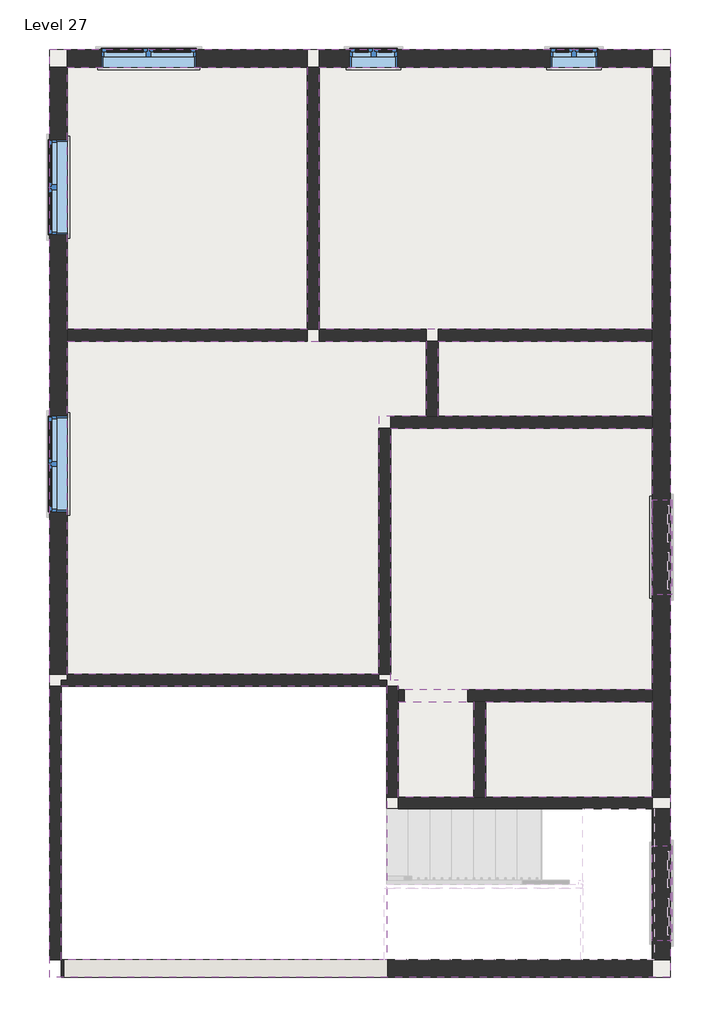
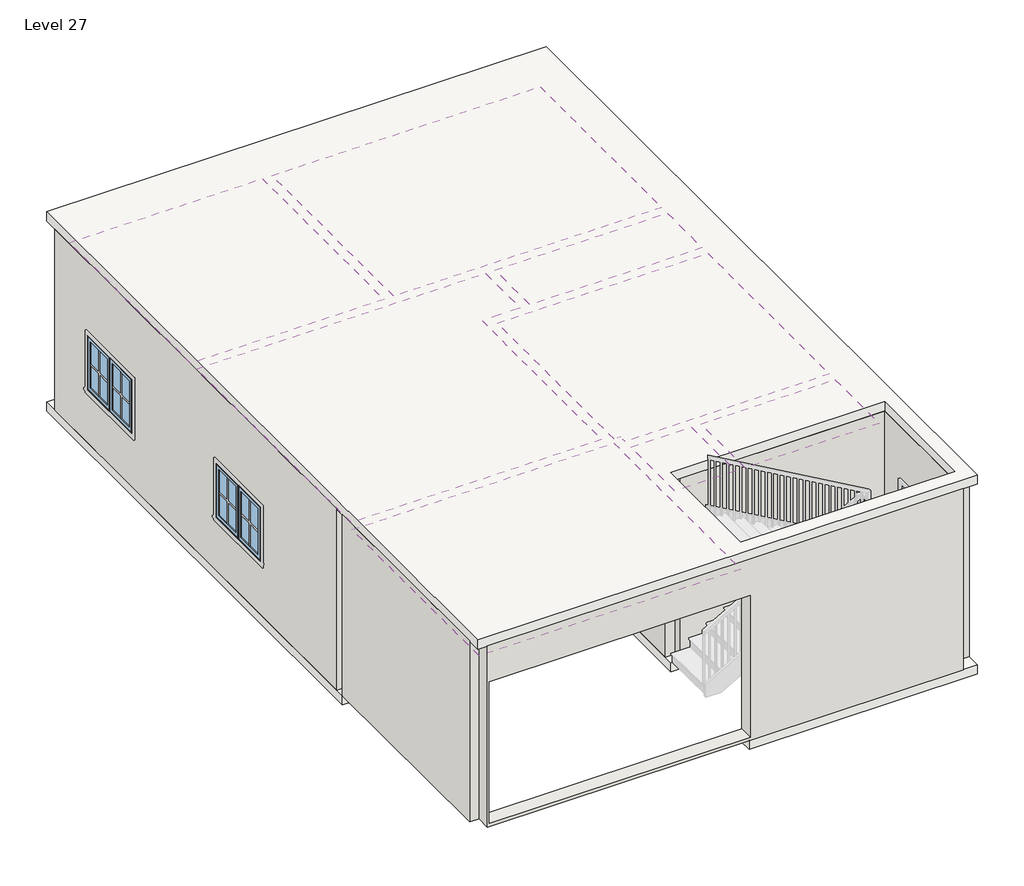
# One storey, part 1 of 3: 27 walls, 11 windows, 8 coverings, 2 slabs.
"""IFC4 building model written with IfcOpenShell, lengths in millimetres."""

from ifc_helpers import new_model, si_unit, frame, origin, place, context, project, spatial, polyline, outline, extrude, faceted_brep, transform, mapped, element, save
from components import window_casement_double_3_c417fced, window_casement_double_4_c19c33cb

model = new_model("IFC4")

# Units and contexts
model_context = context("Model", 3, world=origin())
ifc_project = project(units=[si_unit("LENGTHUNIT", "METRE", prefix="MILLI")], contexts=[model_context])

# Site, building, storey
site = spatial("IfcSite", under=ifc_project)
building = spatial("IfcBuilding", under=site)
storey = spatial("IfcBuildingStorey", under=building, Name="Level 27", Elevation=22402.8)

# Coverings
placement = place(None, origin())
element("IfcCovering", 1, ObjectType="2' x 4' ACT System", at=placement, inside=storey, context=model_context, shape_type="SweptSolid", body=[
    extrude(outline(polyline([(-5680.5154463, 2323.8455275), (-5680.5154463, 5678.2330275), (-2607.1154463, 5678.2330275), (-2607.1154463, 2323.8455275), (-5680.5154463, 2323.8455275)])), frame((0.0, 0.0, 25146.0), z_axis=(0.0, 0.0, 1.0), x_axis=(1.0, 0.0, 0.0)), (0.0, 0.0, 1.0), 57.15),
])
element("IfcCovering", 2, ObjectType="2' x 4' ACT System", at=placement, inside=storey, context=model_context, shape_type="SweptSolid", body=[
    extrude(outline(polyline([(-2454.7154463, 2323.8455275), (-2454.7154463, 5678.2330275), (1812.4845537, 5678.2330275), (1812.4845537, 2323.8455275), (-2454.7154463, 2323.8455275)])), frame((0.0, 0.0, 25146.0), z_axis=(0.0, 0.0, 1.0), x_axis=(1.0, 0.0, 0.0)), (0.0, 0.0, 1.0), 57.15),
])
element("IfcCovering", 3, ObjectType="2' x 4' ACT System", at=placement, inside=storey, context=model_context, shape_type="SweptSolid", body=[
    extrude(outline(polyline([(-5680.5154463, -2095.7544725), (-5680.5154463, 2171.4455275), (-1083.1154463, 2171.4455275), (-1083.1154463, 1206.2455275), (-1692.7154463, 1206.2455275), (-1692.7154463, -2095.7544725), (-5680.5154463, -2095.7544725)])), frame((0.0, 0.0, 25146.0), z_axis=(0.0, 0.0, 1.0), x_axis=(1.0, 0.0, 0.0)), (0.0, 0.0, 1.0), 57.15),
])
element("IfcCovering", 4, ObjectType="2' x 4' ACT System", at=placement, inside=storey, context=model_context, shape_type="SweptSolid", body=[
    extrude(outline(polyline([(-930.7154463, 2171.4455275), (1812.4845537, 2171.4455275), (1812.4845537, 1206.2455275), (-930.7154463, 1206.2455275), (-930.7154463, 2171.4455275)])), frame((0.0, 0.0, 25146.0), z_axis=(0.0, 0.0, 1.0), x_axis=(1.0, 0.0, 0.0)), (0.0, 0.0, 1.0), 57.15),
])
element("IfcCovering", 5, ObjectType="2' x 4' ACT System", at=placement, inside=storey, context=model_context, shape_type="SweptSolid", body=[
    extrude(outline(polyline([(1812.4845537, 1053.8455275), (1812.4845537, -2298.9544725), (-1438.7154463, -2298.9544725), (-1438.7154463, -2171.9544725), (-1540.3154463, -2171.9544725), (-1540.3154463, 1053.8455275), (1812.4845537, 1053.8455275)])), frame((0.0, 0.0, 25146.0), z_axis=(0.0, 0.0, 1.0), x_axis=(1.0, 0.0, 0.0)), (0.0, 0.0, 1.0), 57.15),
])
element("IfcCovering", 6, ObjectType="2' x 4' ACT System", at=placement, inside=storey, context=model_context, shape_type="SweptSolid", body=[
    extrude(outline(polyline([(1812.4845537, -2451.3544725), (1812.4845537, -3670.5544725), (-321.1154463, -3670.5544725), (-321.1154463, -2451.3544725), (1812.4845537, -2451.3544725)])), frame((0.0, 0.0, 25146.0), z_axis=(0.0, 0.0, 1.0), x_axis=(1.0, 0.0, 0.0)), (0.0, 0.0, 1.0), 57.15),
])
element("IfcCovering", 7, ObjectType="2' x 4' ACT System", at=placement, inside=storey, context=model_context, shape_type="SweptSolid", body=[
    extrude(outline(polyline([(-473.5154463, -2451.3544725), (-473.5154463, -3670.5544725), (-1438.7154463, -3670.5544725), (-1438.7154463, -2451.3544725), (-473.5154463, -2451.3544725)])), frame((0.0, 0.0, 25146.0), z_axis=(0.0, 0.0, 1.0), x_axis=(1.0, 0.0, 0.0)), (0.0, 0.0, 1.0), 57.15),
])
element("IfcCovering", 8, ObjectType="2' x 4' ACT System", at=placement, inside=storey, context=model_context, shape_type="SweptSolid", body=[
    extrude(outline(polyline([(-1591.1154463, -2248.1544725), (-1591.1154463, -5753.3544725), (-5756.7154463, -5753.3544725), (-5756.7154463, -2248.1544725), (-1591.1154463, -2248.1544725)])), frame((0.0, 0.0, 25146.0), z_axis=(0.0, 0.0, 1.0), x_axis=(1.0, 0.0, 0.0)), (0.0, 0.0, 1.0), 57.15),
])

# Slabs
element("IfcSlab", 9, ObjectType="Generic - 6\"", at=placement, inside=storey, context=model_context, shape_type="SweptSolid", body=[
    extrude(outline(polyline([(-5909.1154463, -2248.1544725), (-5909.1154463, 5906.8330275), (2041.0845537, 5906.8330275), (2041.0845537, -5981.9544725), (-1591.1154463, -5981.9544725), (-1591.1154463, -5753.3544725), (1812.4845537, -5753.3544725), (1812.4845537, -3822.9544725), (-1591.1154463, -3822.9544725), (-1591.1154463, -2248.1544725), (-5756.7154463, -2248.1544725), (-5909.1154463, -2248.1544725)])), frame((0.0, 0.0, 22250.4), z_axis=(0.0, 0.0, 1.0), x_axis=(1.0, 0.0, 0.0)), (0.0, 0.0, 1.0), 152.4),
])
element("IfcSlab", 10, ObjectType="Generic - 6\"", at=placement, inside=storey, context=model_context, shape_type="SweptSolid", body=[
    extrude(outline(polyline([(2041.0845537, 5906.8330275), (2041.0845537, -5981.9544725), (-5909.1154463, -5981.9544725), (-5909.1154463, 5906.8330275), (2041.0845537, 5906.8330275)]), holes=[polyline([(1812.4845537, -3822.9544725), (-1591.1154463, -3822.9544725), (-1591.1154463, -5753.3544725), (1812.4845537, -5753.3544725), (1812.4845537, -3822.9544725)])]), frame((0.0, 0.0, 25450.8), z_axis=(0.0, 0.0, 1.0), x_axis=(1.0, 0.0, 0.0)), (0.0, 0.0, 1.0), 152.4),
])

# Walls
element("IfcWall", 11, ObjectType="Generic - 6\"", at=placement, inside=storey, context=model_context, shape_type="SweptSolid", body=[
    extrude(outline(polyline([(-5909.1154463, -5753.3544725), (-5909.1154463, -2248.1544725), (-5756.7154463, -2248.1544725), (-5756.7154463, -5753.3544725), (-5909.1154463, -5753.3544725)])), frame((0.0, 0.0, 22402.8), z_axis=(0.0, 0.0, 1.0), x_axis=(1.0, 0.0, 0.0)), (0.0, 0.0, 1.0), 3048.0),
])
element("IfcWall", 12, ObjectType="Generic - 6\"", at=placement, inside=storey, context=model_context, shape_type="Brep", body=[
    faceted_brep([(1812.4845537, -3670.5544725, 22402.8), (-321.1154463, -3670.5544725, 22402.8), (-473.5154463, -3670.5544725, 22402.8), (-1438.7154463, -3670.5544725, 22402.8), (-1438.7154463, -3670.5544725, 25450.8), (-473.5154463, -3670.5544725, 25450.8), (-321.1154463, -3670.5544725, 25450.8), (1812.4845537, -3670.5544725, 25450.8), (1812.4845537, -3822.9544725, 22402.8), (1812.4845537, -3822.9544725, 25450.8), (-1438.7154463, -3822.9544725, 25450.8), (-1438.7154463, -3822.9544725, 22402.8), (1812.4845537, -3746.7544725, 22402.8), (1812.4845537, -3746.7544725, 25450.8)], [[[0, 1, 2, 3, 4, 5, 6, 7]], [[8, 9, 10, 11]], [[3, 2, 1, 0, 12, 8, 11]], [[7, 6, 5, 4, 10, 9, 13]], [[4, 3, 11, 10]], [[0, 7, 13, 9, 8, 12]]]),
])
element("IfcWall", 13, ObjectType="Generic - 6\"", at=placement, inside=storey, context=model_context, shape_type="Brep", body=[
    faceted_brep([(-1438.7154463, -3670.5544725, 22402.8), (-1438.7154463, -2451.3544725, 22402.8), (-1438.7154463, -2298.9544725, 22402.8), (-1438.7154463, -2248.1544725, 22402.8), (-1438.7154463, -2248.1544725, 25450.8), (-1438.7154463, -2298.9544725, 25450.8), (-1438.7154463, -2451.3544725, 25450.8), (-1438.7154463, -3670.5544725, 25450.8), (-1591.1154463, -3670.5544725, 22402.8), (-1591.1154463, -3670.5544725, 25450.8), (-1591.1154463, -2248.1544725, 25450.8), (-1591.1154463, -2248.1544725, 22402.8)], [[[0, 1, 2, 3, 4, 5, 6, 7]], [[8, 9, 10, 11]], [[3, 2, 1, 0, 8, 11]], [[7, 6, 5, 4, 10, 9]], [[0, 7, 9, 8]], [[4, 3, 11, 10]]]),
])
element("IfcWall", 14, ObjectType="Generic - 6\"", at=placement, inside=storey, context=model_context, shape_type="SweptSolid", body=[
    extrude(outline(polyline([(-5680.5154463, -2095.7544725), (-1692.7154463, -2095.7544725), (-1692.7154463, -2171.9544725), (-1591.1154463, -2171.9544725), (-1591.1154463, -2248.1544725), (-5756.7154463, -2248.1544725), (-5756.7154463, -2171.9544725), (-5680.5154463, -2171.9544725), (-5680.5154463, -2095.7544725)])), frame((0.0, 0.0, 22402.8), z_axis=(0.0, 0.0, 1.0), x_axis=(1.0, 0.0, 0.0)), (0.0, 0.0, 1.0), 3048.0),
])
element("IfcWall", 15, ObjectType="Generic - 6\"", at=placement, inside=storey, context=model_context, shape_type="Brep", body=[
    faceted_brep([(1812.4845537, -2451.3544725, 22402.8), (1812.4845537, -2451.3544725, 25450.8), (-321.1154463, -2451.3544725, 25450.8), (-473.5154463, -2451.3544725, 25450.8), (-1438.7154463, -2451.3544725, 25450.8), (-1438.7154463, -2451.3544725, 22402.8), (-1367.0206652, -2451.3544725, 22402.8), (-1367.0206652, -2451.3544725, 24841.2), (-547.4818767, -2451.3544725, 24841.2), (-547.4818767, -2451.3544725, 22402.8), (-473.5154463, -2451.3544725, 22402.8), (-321.1154463, -2451.3544725, 22402.8), (1812.4845537, -2298.9544725, 25450.8), (1812.4845537, -2298.9544725, 22402.8), (-547.4818767, -2298.9544725, 22402.8), (-547.4818767, -2298.9544725, 24841.2), (-1367.0206652, -2298.9544725, 24841.2), (-1367.0206652, -2298.9544725, 22402.8), (-1438.7154463, -2298.9544725, 22402.8), (-1438.7154463, -2298.9544725, 25450.8)], [[[0, 1, 2, 3, 4, 5, 6, 7, 8, 9, 10, 11]], [[12, 13, 14, 15, 16, 17, 18, 19]], [[5, 18, 17, 6]], [[13, 0, 11, 10, 9, 14]], [[4, 3, 2, 1, 12, 19]], [[1, 0, 13, 12]], [[5, 4, 19, 18]], [[7, 16, 15, 8]], [[16, 7, 6, 17]], [[8, 15, 14, 9]]]),
])
element("IfcWall", 16, ObjectType="Generic - 6\"", at=placement, inside=storey, context=model_context, shape_type="SweptSolid", body=[
    extrude(outline(polyline([(-321.1154463, -2451.3544725), (-321.1154463, -3670.5544725), (-473.5154463, -3670.5544725), (-473.5154463, -2451.3544725), (-321.1154463, -2451.3544725)])), frame((0.0, 0.0, 22402.8), z_axis=(0.0, 0.0, 1.0), x_axis=(1.0, 0.0, 0.0)), (0.0, 0.0, 1.0), 3048.0),
])
element("IfcWall", 17, ObjectType="Generic - 6\"", at=placement, inside=storey, context=model_context, shape_type="Brep", body=[
    faceted_brep([(-1540.3154463, -2095.7544725, 22402.8), (-1540.3154463, 1053.8455275, 22402.8), (-1540.3154463, 1053.8455275, 25450.8), (-1540.3154463, -2095.7544725, 25450.8), (-1692.7154463, -2095.7544725, 22402.8), (-1692.7154463, -2095.7544725, 25450.8), (-1692.7154463, 1053.8455275, 25450.8), (-1692.7154463, 1053.8455275, 22402.8), (-1591.1154463, -2095.7544725, 22402.8), (-1591.1154463, -2095.7544725, 25450.8)], [[[0, 1, 2, 3]], [[4, 5, 6, 7]], [[1, 0, 8, 4, 7]], [[3, 2, 6, 5, 9]], [[0, 3, 9, 5, 4, 8]], [[2, 1, 7, 6]]]),
])
element("IfcWall", 18, ObjectType="Generic - 6\"", at=placement, inside=storey, context=model_context, shape_type="Brep", body=[
    faceted_brep([(-1540.3154463, 1053.8455275, 22402.8), (1812.4845537, 1053.8455275, 22402.8), (1812.4845537, 1053.8455275, 25450.8), (-1540.3154463, 1053.8455275, 25450.8), (-1540.3154463, 1206.2455275, 22402.8), (-1540.3154463, 1206.2455275, 25450.8), (-1083.1154463, 1206.2455275, 25450.8), (-930.7154463, 1206.2455275, 25450.8), (1812.4845537, 1206.2455275, 25450.8), (1812.4845537, 1206.2455275, 22402.8), (-930.7154463, 1206.2455275, 22402.8), (-1083.1154463, 1206.2455275, 22402.8)], [[[0, 1, 2, 3]], [[4, 5, 6, 7, 8, 9, 10, 11]], [[1, 0, 4, 11, 10, 9]], [[3, 2, 8, 7, 6, 5]], [[2, 1, 9, 8]], [[0, 3, 5, 4]]]),
])
element("IfcWall", 19, ObjectType="Generic - 6\"", at=placement, inside=storey, context=model_context, shape_type="Brep", body=[
    faceted_brep([(-930.7154463, 1206.2455275, 22402.8), (-930.7154463, 2171.4455275, 22402.8), (-930.7154463, 2171.4455275, 25450.8), (-930.7154463, 1206.2455275, 25450.8), (-1083.1154463, 1206.2455275, 22402.8), (-1083.1154463, 1206.2455275, 25450.8), (-1083.1154463, 2171.4455275, 25450.8), (-1083.1154463, 2171.4455275, 22402.8), (-1006.9154463, 2171.4455275, 22402.8), (-1006.9154463, 2171.4455275, 25450.8)], [[[0, 1, 2, 3]], [[4, 5, 6, 7]], [[1, 0, 4, 7, 8]], [[3, 2, 9, 6, 5]], [[0, 3, 5, 4]], [[2, 1, 8, 7, 6, 9]]]),
])
element("IfcWall", 20, ObjectType="Generic - 6\"", at=placement, inside=storey, context=model_context, shape_type="SweptSolid", body=[
    extrude(outline(polyline([(-930.7154463, 2323.8455275), (1812.4845537, 2323.8455275), (1812.4845537, 2171.4455275), (-930.7154463, 2171.4455275), (-930.7154463, 2323.8455275)])), frame((0.0, 0.0, 22402.8), z_axis=(0.0, 0.0, 1.0), x_axis=(1.0, 0.0, 0.0)), (0.0, 0.0, 1.0), 3048.0),
])
element("IfcWall", 21, ObjectType="Generic - 6\"", at=placement, inside=storey, context=model_context, shape_type="Brep", body=[
    faceted_brep([(-2607.1154463, 5678.2330275, 22402.8), (-2607.1154463, 2323.8455275, 22402.8), (-2607.1154463, 2323.8455275, 25450.8), (-2607.1154463, 5678.2330275, 25450.8), (-2454.7154463, 5678.2330275, 22402.8), (-2454.7154463, 5678.2330275, 25450.8), (-2454.7154463, 2323.8455275, 25450.8), (-2454.7154463, 2323.8455275, 22402.8), (-2530.9154463, 5678.2330275, 22402.8), (-2530.9154463, 2323.8455275, 22402.8), (-2530.9154463, 2323.8455275, 25450.8), (-2530.9154463, 5678.2330275, 25450.8)], [[[0, 1, 2, 3]], [[4, 5, 6, 7]], [[1, 0, 8, 4, 7, 9]], [[3, 2, 10, 6, 5, 11]], [[0, 3, 11, 5, 4, 8]], [[2, 1, 9, 7, 6, 10]]]),
])
element("IfcWall", 22, ObjectType="Generic - 6\"", at=placement, inside=storey, context=model_context, shape_type="SweptSolid", body=[
    extrude(outline(polyline([(-5680.5154463, 2323.8455275), (-2607.1154463, 2323.8455275), (-2607.1154463, 2171.4455275), (-5680.5154463, 2171.4455275), (-5680.5154463, 2323.8455275)])), frame((0.0, 0.0, 22402.8), z_axis=(0.0, 0.0, 1.0), x_axis=(1.0, 0.0, 0.0)), (0.0, 0.0, 1.0), 3048.0),
])
element("IfcWall", 23, ObjectType="Generic - 6\"", at=placement, inside=storey, context=model_context, shape_type="SweptSolid", body=[
    extrude(outline(polyline([(-2454.7154463, 2323.8455275), (-1083.1154463, 2323.8455275), (-1083.1154463, 2171.4455275), (-2454.7154463, 2171.4455275), (-2454.7154463, 2323.8455275)])), frame((0.0, 0.0, 22402.8), z_axis=(0.0, 0.0, 1.0), x_axis=(1.0, 0.0, 0.0)), (0.0, 0.0, 1.0), 3048.0),
])
element("IfcWall", 24, ObjectType="Generic - 6\"", at=placement, inside=storey, context=model_context, shape_type="SweptSolid", body=[
    extrude(outline(polyline([(-5680.5154463, -2095.7544725), (-1692.7154463, -2095.7544725), (-1692.7154463, -2171.9544725), (-1591.1154463, -2171.9544725), (-1591.1154463, -2248.1544725), (-5756.7154463, -2248.1544725), (-5756.7154463, -2171.9544725), (-5680.5154463, -2171.9544725), (-5680.5154463, -2095.7544725)])), frame((0.0, 0.0, 22402.8), z_axis=(0.0, 0.0, 1.0), x_axis=(1.0, 0.0, 0.0)), (0.0, 0.0, 1.0), 3048.0),
])
element("IfcWall", 25, ObjectType="Generic - 6\"", at=placement, inside=storey, context=model_context, shape_type="Brep", body=[
    faceted_brep([(-2607.1154463, 5678.2330275, 22402.8), (-2607.1154463, 2323.8455275, 22402.8), (-2607.1154463, 2323.8455275, 25450.8), (-2607.1154463, 5678.2330275, 25450.8), (-2454.7154463, 5678.2330275, 22402.8), (-2454.7154463, 5678.2330275, 25450.8), (-2454.7154463, 2323.8455275, 25450.8), (-2454.7154463, 2323.8455275, 22402.8), (-2530.9154463, 5678.2330275, 22402.8), (-2530.9154463, 2323.8455275, 22402.8), (-2530.9154463, 2323.8455275, 25450.8), (-2530.9154463, 5678.2330275, 25450.8)], [[[0, 1, 2, 3]], [[4, 5, 6, 7]], [[1, 0, 8, 4, 7, 9]], [[3, 2, 10, 6, 5, 11]], [[0, 3, 11, 5, 4, 8]], [[2, 1, 9, 7, 6, 10]]]),
])
element("IfcWall", 26, ObjectType="Generic - 6\"", at=placement, inside=storey, context=model_context, shape_type="SweptSolid", body=[
    extrude(outline(polyline([(-5680.5154463, 2323.8455275), (-2607.1154463, 2323.8455275), (-2607.1154463, 2171.4455275), (-5680.5154463, 2171.4455275), (-5680.5154463, 2323.8455275)])), frame((0.0, 0.0, 22402.8), z_axis=(0.0, 0.0, 1.0), x_axis=(1.0, 0.0, 0.0)), (0.0, 0.0, 1.0), 3048.0),
])
element("IfcWall", 27, ObjectType="Generic - 6\"", at=placement, inside=storey, context=model_context, shape_type="SweptSolid", body=[
    extrude(outline(polyline([(-2454.7154463, 2323.8455275), (-1083.1154463, 2323.8455275), (-1083.1154463, 2171.4455275), (-2454.7154463, 2171.4455275), (-2454.7154463, 2323.8455275)])), frame((0.0, 0.0, 22402.8), z_axis=(0.0, 0.0, 1.0), x_axis=(1.0, 0.0, 0.0)), (0.0, 0.0, 1.0), 3048.0),
])
element("IfcWall", 28, ObjectType="Generic - 9\"", at=placement, inside=storey, context=model_context, shape_type="SweptSolid", body=[
    extrude(outline(polyline([(22402.8, -5680.5154463), (22402.8, -2607.1154463), (25450.8, -2607.1154463), (25450.8, -5680.5154463), (22402.8, -5680.5154463)]), holes=[polyline([(24231.6, -4029.5154463), (23317.2, -4029.5154463), (23317.2, -5248.7154463), (24231.6, -5248.7154463), (24231.6, -4029.5154463)])]), frame((0.0, 5678.2330275, 0.0), z_axis=(0.0, 1.0, 0.0), x_axis=(0.0, 0.0, 1.0)), (0.0, 0.0, 1.0), 228.6),
])
element("IfcWall", 29, ObjectType="Generic - 9\"", at=placement, inside=storey, context=model_context, shape_type="Brep", body=[
    faceted_brep([(1812.4845537, 5678.2330275, 22402.8), (1812.4845537, 2323.8455275, 22402.8), (1812.4845537, 2171.4455275, 22402.8), (1812.4845537, 1206.2455275, 22402.8), (1812.4845537, 1053.8455275, 22402.8), (1812.4845537, -2298.9544725, 22402.8), (1812.4845537, -2451.3544725, 22402.8), (1812.4845537, -3670.5544725, 22402.8), (1812.4845537, -3670.5544725, 25450.8), (1812.4845537, -2451.3544725, 25450.8), (1812.4845537, -2298.9544725, 25450.8), (1812.4845537, 1053.8455275, 25450.8), (1812.4845537, 1206.2455275, 25450.8), (1812.4845537, 2171.4455275, 25450.8), (1812.4845537, 2323.8455275, 25450.8), (1812.4845537, 5678.2330275, 25450.8), (1812.4845537, -1079.7544725, 24536.4), (1812.4845537, -1079.7544725, 23622.0), (1812.4845537, 139.4455275, 23622.0), (1812.4845537, 139.4455275, 24536.4), (2041.0845537, 5678.2330275, 22402.8), (2041.0845537, 5678.2330275, 25450.8), (2041.0845537, -3670.5544725, 25450.8), (2041.0845537, -3670.5544725, 22402.8), (2041.0845537, -1079.7544725, 24536.4), (2041.0845537, 139.4455275, 24536.4), (2041.0845537, 139.4455275, 23622.0), (2041.0845537, -1079.7544725, 23622.0)], [[[0, 1, 2, 3, 4, 5, 6, 7, 8, 9, 10, 11, 12, 13, 14, 15], [16, 17, 18, 19]], [[20, 21, 22, 23], [24, 25, 26, 27]], [[7, 6, 5, 4, 3, 2, 1, 0, 20, 23]], [[15, 14, 13, 12, 11, 10, 9, 8, 22, 21]], [[17, 16, 24, 27]], [[18, 17, 27, 26]], [[19, 18, 26, 25]], [[16, 19, 25, 24]], [[0, 15, 21, 20]], [[8, 7, 23, 22]]]),
])
element("IfcWall", 30, ObjectType="Generic - 9\"", at=placement, inside=storey, context=model_context, shape_type="SweptSolid", body=[
    extrude(outline(polyline([(22402.8, -5756.7154463), (22402.8, 1812.4845537), (25450.8, 1812.4845537), (25450.8, -5756.7154463), (22402.8, -5756.7154463)]), holes=[polyline([(24841.2, -5729.1673724), (24841.2, -1576.8982041), (22453.6, -1576.8982041), (22453.6, -5729.1673724), (24841.2, -5729.1673724)])]), frame((0.0, -5981.9544725, 0.0), z_axis=(0.0, 1.0, 0.0), x_axis=(0.0, 0.0, 1.0)), (0.0, 0.0, 1.0), 228.6),
])
element("IfcWall", 31, ObjectType="Generic - 9\"", at=placement, inside=storey, context=model_context, shape_type="Brep", body=[
    faceted_brep([(-5909.1154463, 5678.2330275, 22402.8), (-5909.1154463, -2095.7544725, 22402.8), (-5909.1154463, -2095.7544725, 25450.8), (-5909.1154463, 5678.2330275, 25450.8), (-5909.1154463, 4751.1330275, 24231.6), (-5909.1154463, 3531.9330275, 24231.6), (-5909.1154463, 3531.9330275, 23317.2), (-5909.1154463, 4751.1330275, 23317.2), (-5909.1154463, 1206.2455275, 24231.6), (-5909.1154463, -12.9544725, 24231.6), (-5909.1154463, -12.9544725, 23317.2), (-5909.1154463, 1206.2455275, 23317.2), (-5680.5154463, 5678.2330275, 22402.8), (-5680.5154463, 5678.2330275, 25450.8), (-5680.5154463, 2323.8455275, 25450.8), (-5680.5154463, 2171.4455275, 25450.8), (-5680.5154463, -2095.7544725, 25450.8), (-5680.5154463, -2095.7544725, 22402.8), (-5680.5154463, 2171.4455275, 22402.8), (-5680.5154463, 2323.8455275, 22402.8), (-5680.5154463, 4751.1330275, 24231.6), (-5680.5154463, 4751.1330275, 23317.2), (-5680.5154463, 3531.9330275, 23317.2), (-5680.5154463, 3531.9330275, 24231.6), (-5680.5154463, 1206.2455275, 24231.6), (-5680.5154463, 1206.2455275, 23317.2), (-5680.5154463, -12.9544725, 23317.2), (-5680.5154463, -12.9544725, 24231.6)], [[[0, 1, 2, 3], [4, 5, 6, 7], [8, 9, 10, 11]], [[12, 13, 14, 15, 16, 17, 18, 19], [20, 21, 22, 23], [24, 25, 26, 27]], [[1, 0, 12, 19, 18, 17]], [[3, 2, 16, 15, 14, 13]], [[21, 20, 4, 7]], [[22, 21, 7, 6]], [[23, 22, 6, 5]], [[20, 23, 5, 4]], [[25, 24, 8, 11]], [[26, 25, 11, 10]], [[27, 26, 10, 9]], [[24, 27, 9, 8]], [[0, 3, 13, 12]], [[2, 1, 17, 16]]]),
])
element("IfcWall", 32, ObjectType="Generic - 9\"", at=placement, inside=storey, context=model_context, shape_type="SweptSolid", body=[
    extrude(outline(polyline([(22402.8, -2454.7154463), (22402.8, 1812.4845537), (25450.8, 1812.4845537), (25450.8, -2454.7154463), (22402.8, -2454.7154463)]), holes=[polyline([(24231.6, -1451.4154463), (23317.2, -1451.4154463), (23317.2, -2061.0154463), (24231.6, -2061.0154463), (24231.6, -1451.4154463)]), polyline([(24231.6, 1113.9845537), (23317.2, 1113.9845537), (23317.2, 504.3845537), (24231.6, 504.3845537), (24231.6, 1113.9845537)])]), frame((0.0, 5678.2330275, 0.0), z_axis=(0.0, 1.0, 0.0), x_axis=(0.0, 0.0, 1.0)), (0.0, 0.0, 1.0), 228.6),
])
element("IfcWall", 33, ObjectType="Generic - 9\"", at=placement, inside=storey, context=model_context, shape_type="SweptSolid", body=[
    extrude(outline(polyline([(-3822.9544725, 22402.8), (-5753.3544725, 22402.8), (-5753.3544725, 25450.8), (-3822.9544725, 25450.8), (-3822.9544725, 22402.8)]), holes=[polyline([(-5512.0544725, 24536.4), (-5512.0544725, 23622.0), (-4292.8544725, 23622.0), (-4292.8544725, 24536.4), (-5512.0544725, 24536.4)])]), frame((1812.4845537, 0.0, 0.0), z_axis=(1.0, 0.0, 0.0), x_axis=(0.0, 1.0, 0.0)), (0.0, 0.0, 1.0), 228.6),
])
element("IfcWall", 34, ObjectType="Generic - 9\"", at=placement, inside=storey, context=model_context, shape_type="SweptSolid", body=[
    extrude(outline(polyline([(22402.8, -5680.5154463), (22402.8, -2607.1154463), (25450.8, -2607.1154463), (25450.8, -5680.5154463), (22402.8, -5680.5154463)]), holes=[polyline([(24231.6, -4029.5154463), (23317.2, -4029.5154463), (23317.2, -5248.7154463), (24231.6, -5248.7154463), (24231.6, -4029.5154463)])]), frame((0.0, 5678.2330275, 0.0), z_axis=(0.0, 1.0, 0.0), x_axis=(0.0, 0.0, 1.0)), (0.0, 0.0, 1.0), 228.6),
])
element("IfcWall", 35, ObjectType="Generic - 9\"", at=placement, inside=storey, context=model_context, shape_type="SweptSolid", body=[
    extrude(outline(polyline([(22402.8, -5756.7154463), (22402.8, 1812.4845537), (25450.8, 1812.4845537), (25450.8, -5756.7154463), (22402.8, -5756.7154463)]), holes=[polyline([(24841.2, -5729.1673724), (24841.2, -1576.8982041), (22453.6, -1576.8982041), (22453.6, -5729.1673724), (24841.2, -5729.1673724)])]), frame((0.0, -5981.9544725, 0.0), z_axis=(0.0, 1.0, 0.0), x_axis=(0.0, 0.0, 1.0)), (0.0, 0.0, 1.0), 228.6),
])
element("IfcWall", 36, ObjectType="Generic - 9\"", at=placement, inside=storey, context=model_context, shape_type="SweptSolid", body=[
    extrude(outline(polyline([(22402.8, -2454.7154463), (22402.8, 1812.4845537), (25450.8, 1812.4845537), (25450.8, -2454.7154463), (22402.8, -2454.7154463)]), holes=[polyline([(24231.6, -1451.4154463), (23317.2, -1451.4154463), (23317.2, -2061.0154463), (24231.6, -2061.0154463), (24231.6, -1451.4154463)]), polyline([(24231.6, 1113.9845537), (23317.2, 1113.9845537), (23317.2, 504.3845537), (24231.6, 504.3845537), (24231.6, 1113.9845537)])]), frame((0.0, 5678.2330275, 0.0), z_axis=(0.0, 1.0, 0.0), x_axis=(0.0, 0.0, 1.0)), (0.0, 0.0, 1.0), 228.6),
])
element("IfcWall", 37, ObjectType="Generic - 9\"", at=placement, inside=storey, context=model_context, shape_type="SweptSolid", body=[
    extrude(outline(polyline([(-3822.9544725, 22402.8), (-5753.3544725, 22402.8), (-5753.3544725, 25450.8), (-3822.9544725, 25450.8), (-3822.9544725, 22402.8)]), holes=[polyline([(-5512.0544725, 24536.4), (-5512.0544725, 23622.0), (-4292.8544725, 23622.0), (-4292.8544725, 24536.4), (-5512.0544725, 24536.4)])]), frame((1812.4845537, 0.0, 0.0), z_axis=(1.0, 0.0, 0.0), x_axis=(0.0, 1.0, 0.0)), (0.0, 0.0, 1.0), 228.6),
])

# Windows
window_casement_double_3_shape = window_casement_double_3_c417fced(model_context)
element("IfcWindow", 38, ObjectType="Window-Casement-Double : 3'", at=placement, inside=storey, context=model_context, shape_type="MappedRepresentation", body=[
    mapped(window_casement_double_3_shape, transform((-1756.2154463, 5792.5330275, 22402.8), x_axis=(1.0, 0.0, 0.0), y_axis=(0.0, 1.0, 0.0), z_axis=(0.0, 0.0, 1.0))),
])
element("IfcWindow", 39, ObjectType="Window-Casement-Double : 3'", at=placement, inside=storey, context=model_context, shape_type="MappedRepresentation", body=[
    mapped(window_casement_double_3_shape, transform((809.1845537, 5792.5330275, 22402.8), x_axis=(1.0, 0.0, 0.0), y_axis=(0.0, 1.0, 0.0), z_axis=(0.0, 0.0, 1.0))),
])
element("IfcWindow", 40, ObjectType="Window-Casement-Double : 3'", at=placement, inside=storey, context=model_context, shape_type="MappedRepresentation", body=[
    mapped(window_casement_double_3_shape, transform((-1756.2154463, 5792.5330275, 22402.8), x_axis=(1.0, 0.0, 0.0), y_axis=(0.0, 1.0, 0.0), z_axis=(0.0, 0.0, 1.0))),
])
element("IfcWindow", 41, ObjectType="Window-Casement-Double : 3'", at=placement, inside=storey, context=model_context, shape_type="MappedRepresentation", body=[
    mapped(window_casement_double_3_shape, transform((809.1845537, 5792.5330275, 22402.8), x_axis=(1.0, 0.0, 0.0), y_axis=(0.0, 1.0, 0.0), z_axis=(0.0, 0.0, 1.0))),
])
window_casement_double_4_shape = window_casement_double_4_c19c33cb(model_context)
element("IfcWindow", 42, ObjectType="Window-Casement-Double : 4'", at=placement, inside=storey, context=model_context, shape_type="MappedRepresentation", body=[
    mapped(window_casement_double_4_shape, transform((-4639.1154463, 5792.5330275, 22402.8), x_axis=(1.0, 0.0, 0.0), y_axis=(0.0, 1.0, 0.0), z_axis=(0.0, 0.0, 1.0))),
])
element("IfcWindow", 43, ObjectType="Window-Casement-Double : 4'", at=placement, inside=storey, context=model_context, shape_type="MappedRepresentation", body=[
    mapped(window_casement_double_4_shape, transform((-5794.8154463, 4141.5330275, 22402.8), x_axis=(0.0, 1.0, 0.0), y_axis=(-1.0, 0.0, 0.0), z_axis=(0.0, 0.0, 1.0))),
])
element("IfcWindow", 44, ObjectType="Window-Casement-Double : 4'", at=placement, inside=storey, context=model_context, shape_type="MappedRepresentation", body=[
    mapped(window_casement_double_4_shape, transform((-5794.8154463, 596.6455275, 22402.8), x_axis=(0.0, 1.0, 0.0), y_axis=(-1.0, 0.0, 0.0), z_axis=(0.0, 0.0, 1.0))),
])
element("IfcWindow", 45, ObjectType="Window-Casement-Double : 4'", at=placement, inside=storey, context=model_context, shape_type="MappedRepresentation", body=[
    mapped(window_casement_double_4_shape, transform((1926.7845537, -470.1544725, 22707.6), x_axis=(0.0, -1.0, 0.0), y_axis=(1.0, 0.0, 0.0), z_axis=(0.0, 0.0, 1.0))),
])
element("IfcWindow", 46, ObjectType="Window-Casement-Double : 4'", at=placement, inside=storey, context=model_context, shape_type="MappedRepresentation", body=[
    mapped(window_casement_double_4_shape, transform((1926.7845537, -4902.4544725, 22707.6), x_axis=(0.0, -1.0, 0.0), y_axis=(1.0, 0.0, 0.0), z_axis=(0.0, 0.0, 1.0))),
])
element("IfcWindow", 47, ObjectType="Window-Casement-Double : 4'", at=placement, inside=storey, context=model_context, shape_type="MappedRepresentation", body=[
    mapped(window_casement_double_4_shape, transform((-4639.1154463, 5792.5330275, 22402.8), x_axis=(1.0, 0.0, 0.0), y_axis=(0.0, 1.0, 0.0), z_axis=(0.0, 0.0, 1.0))),
])
element("IfcWindow", 48, ObjectType="Window-Casement-Double : 4'", at=placement, inside=storey, context=model_context, shape_type="MappedRepresentation", body=[
    mapped(window_casement_double_4_shape, transform((1926.7845537, -4902.4544725, 22707.6), x_axis=(0.0, -1.0, 0.0), y_axis=(1.0, 0.0, 0.0), z_axis=(0.0, 0.0, 1.0))),
])

save(model, "model.ifc")

# Revit data of these elements
# Type "2' x 4' ACT System"
#   Assembly Code = "C3030210"
#   built-in parameter 1002203 = 1 (stored number, unit not read)
#   built-in parameter 1002202 = 1 (stored number, unit not read)
#   Layers, outside or top first: 0' - 1 5/8" "Default" (function 1); 0' - 0 5/8" "Acoustic Ceiling Tile 24 x 48" (function 5)
# Type "Generic - 6\""
#   Assembly Code = "B1010"
#   Function = 0
#   Layers, outside or top first: 0' - 6" no material (function 1)
# Type "Generic - 6\""
#   Assembly Code = "B2010"
#   Layers, outside or top first: 0' - 6" no material (function 1)
# Type "Generic - 9\""
#   Assembly Code = "B2010"
#   Layers, outside or top first: 0' - 9" no material (function 1)
# Type "Window-Casement-Double : 3'"
#   Type Mark = "19"
#   Fire Rating = "0.5h"
#   Assembly Code = "B2020100"
#   Analytic Construction = "Double glazing - domestic"
#   Frame Extension [instance default] = 0' - 0 1/4"
#   Window Inset [instance default] = 0' - 0"
#   Wall Thickness [instance default] = 0' - 6"
#   Interior Wall Closure [instance default] = 0' - 2 1/4"
#   Half Width = 1' - 0"
#   Visual Light Transmittance = 0.81
#   Thermal Resistance (R) = 1.8146 (h·ft²·°F)/BTU
#   Solar Heat Gain Coefficient = 0.76
#   Rough Width = 2' - 0 1/2"
#   Rough Height = 3' - 0 1/2"
#   Height = 3' - 0"
#   Heat Transfer Coefficient (U) = 0.5511 BTU/(h·ft²·°F)
#   Exterior Wall Closure [instance default] = 0' - 1 1/4"
#   Extension Jamb [instance default] = 0' - 2 1/4"
#   Default Sill Height = 3' - 0"
#   Width = 2' - 0"
#   Muntin Visibility = yes
#   Interior Trim Visibility [instance default] = yes
#   Exterior Trim Visibility [instance default] = yes
#   Extension Jamb Visibility [instance default] = yes
#   Interior Trim Material = Wood - Stained
#   Muntin Pattern = Muntin Pattern_2x2 : Muntin Pattern_2x2
#   Interior Trim = Trim-Window-Interior-Flat : Picture Frame
#   Interior Frame Material = Wood - Stained
#   Glass Panel Material = Glass
#   Exterior Trim Material = Clad - White
#   Exterior Trim = Trim-Window-Exterior-Flat : with Sill
#   Exterior Frame Material = Clad - White
#   Wall Closure = (empty or 0)
# Type "Window-Casement-Double : 4'"
#   Type Mark = "18"
#   Fire Rating = "0.5h"
#   Assembly Code = "B2020100"
#   Analytic Construction = "Double glazing - domestic"
#   Frame Extension [instance default] = 0' - 0 1/4"
#   Window Inset [instance default] = 0' - 0"
#   Wall Thickness [instance default] = 0' - 6"
#   Interior Wall Closure [instance default] = 0' - 2 1/4"
#   Half Width = 2' - 0"
#   Visual Light Transmittance = 0.81
#   Thermal Resistance (R) = 1.8146 (h·ft²·°F)/BTU
#   Solar Heat Gain Coefficient = 0.76
#   Rough Width = 4' - 0 1/2"
#   Rough Height = 3' - 0 1/2"
#   Height = 3' - 0"
#   Heat Transfer Coefficient (U) = 0.5511 BTU/(h·ft²·°F)
#   Exterior Wall Closure [instance default] = 0' - 1 1/4"
#   Extension Jamb [instance default] = 0' - 2 1/4"
#   Default Sill Height = 3' - 0"
#   Width = 4' - 0"
#   Muntin Visibility = yes
#   Interior Trim Visibility [instance default] = yes
#   Exterior Trim Visibility [instance default] = yes
#   Extension Jamb Visibility [instance default] = yes
#   Interior Trim Material = Wood - Stained
#   Muntin Pattern = Muntin Pattern_2x2 : Muntin Pattern_2x2
#   Interior Trim = Trim-Window-Interior-Flat : Picture Frame
#   Interior Frame Material = Wood - Stained
#   Glass Panel Material = Glass
#   Exterior Trim Material = Clad - White
#   Exterior Trim = Trim-Window-Exterior-Flat : with Sill
#   Exterior Frame Material = Clad - White
#   Wall Closure = (empty or 0)
# Elements 1, 2, 3, 4, 5, 6, 7, 8 (IfcCovering, "2' x 4' ACT System")
#   Height Offset From Level = 9' - 0"
#   Phase Created = New Construction
#   Materials on its faces: "Acoustic Ceiling Tile 24 x 48", "Default"
# Element 9 (IfcSlab, "Generic - 6\"")
#   built-in parameter 1001955 = -1.5708 (stored number, unit not read)
#   Height Offset From Level = 0' - 0"
#   Phase Created = New Construction
#   Materials on its faces: "Default Floor", "TILE"
# Element 10 (IfcSlab, "Generic - 6\"")
#   Height Offset From Level = 10' - 6"
#   Phase Created = New Construction
#   Materials on its faces: "Default Floor", "TILE"
# Element 11 (IfcWall, "Generic - 6\"")
#   Top Offset = 0' - 0"
#   Base Offset = 0' - 0"
#   Unconnected Height = 10' - 0"
#   wall height = 10' - 0"
#   Phase Created = New Construction
#   Base Constraint = Level 27
#   Materials on its faces: "Default Wall", "WALL PAINT 4"
# Element 12 (IfcWall, "Generic - 6\"")
#   Top Offset = 0' - 0"
#   Base Offset = 0' - 0"
#   Unconnected Height = 10' - 0"
#   wall height = 10' - 0"
#   Phase Created = New Construction
#   Base Constraint = Level 27
#   Materials on its faces: "Default Wall", "WALL PAINT 5", "MARBLE"
# Element 13 (IfcWall, "Generic - 6\"")
#   Top Offset = 0' - 0"
#   Base Offset = 0' - 0"
#   Unconnected Height = 10' - 0"
#   wall height = 10' - 0"
#   Phase Created = New Construction
#   Base Constraint = Level 27
#   Materials on its faces: "Default Wall", "WALL PAINT 4", "MARBLE"
# Elements 14, 24 (IfcWall, "Generic - 6\"")
#   Top Offset = 0' - 0"
#   Base Offset = 0' - 0"
#   Unconnected Height = 10' - 0"
#   wall height = 10' - 0"
#   Phase Created = New Construction
#   Base Constraint = Level 27
#   Materials on its faces: "Default Wall", "WALL PAINT 2", "MARBLE"
# Elements 15, 18 (IfcWall, "Generic - 6\"")
#   Top Offset = 0' - 0"
#   Base Offset = 0' - 0"
#   Unconnected Height = 10' - 0"
#   wall height = 10' - 0"
#   Phase Created = New Construction
#   Base Constraint = Level 27
#   Materials on its faces: "Default Wall", "WALL PAINT 4", "WALL PAINT 5"
# Element 16 (IfcWall, "Generic - 6\"")
#   Top Offset = 0' - 0"
#   Base Offset = 0' - 0"
#   Unconnected Height = 10' - 0"
#   wall height = 10' - 0"
#   Phase Created = New Construction
#   Base Constraint = Level 27
#   Materials on its faces: "Default Wall", "WALL PAINT 5"
# Element 17 (IfcWall, "Generic - 6\"")
#   Top Offset = 0' - 0"
#   Base Offset = 0' - 0"
#   Unconnected Height = 10' - 0"
#   wall height = 10' - 0"
#   Phase Created = New Construction
#   Base Constraint = Level 27
#   Materials on its faces: "Default Wall", "WALL PAINT 4", "WALL PAINT 2"
# Element 19 (IfcWall, "Generic - 6\"")
#   Top Offset = 0' - 0"
#   Base Offset = 0' - 0"
#   Unconnected Height = 10' - 0"
#   wall height = 10' - 0"
#   Phase Created = New Construction
#   Base Constraint = Level 27
#   Materials on its faces: "Default Wall", "WALL PAINT 5", "WALL PAINT 2"
# Element 20 (IfcWall, "Generic - 6\"")
#   Top Offset = 0' - 0"
#   Base Offset = 0' - 0"
#   Unconnected Height = 10' - 0"
#   wall height = 10' - 0"
#   Phase Created = New Construction
#   Base Constraint = Level 27
#   Materials on its faces: "Default Wall", "WALL PAINT 3", "WALL PAINT 5"
# Elements 21, 25 (IfcWall, "Generic - 6\"")
#   Top Offset = 0' - 0"
#   Base Offset = 0' - 0"
#   Unconnected Height = 10' - 0"
#   wall height = 10' - 0"
#   Phase Created = New Construction
#   Base Constraint = Level 27
#   Materials on its faces: "Default Wall", "WALL PAINT 1", "WALL PAINT 3"
# Elements 22, 26 (IfcWall, "Generic - 6\"")
#   Top Offset = 0' - 0"
#   Base Offset = 0' - 0"
#   Unconnected Height = 10' - 0"
#   wall height = 10' - 0"
#   Phase Created = New Construction
#   Base Constraint = Level 27
#   Materials on its faces: "Default Wall", "WALL PAINT 1", "WALL PAINT 2"
# Elements 23, 27 (IfcWall, "Generic - 6\"")
#   Top Offset = 0' - 0"
#   Base Offset = 0' - 0"
#   Unconnected Height = 10' - 0"
#   wall height = 10' - 0"
#   Phase Created = New Construction
#   Base Constraint = Level 27
#   Materials on its faces: "Default Wall", "WALL PAINT 3", "WALL PAINT 2"
# Elements 28, 34 (IfcWall, "Generic - 9\"")
#   Top Offset = 0' - 0"
#   Base Offset = 0' - 0"
#   Unconnected Height = 10' - 0"
#   wall height = 10' - 0"
#   Phase Created = New Construction
#   Base Constraint = Level 27
#   Materials on its faces: "Default Wall", "WALL PAINT 1"
# Elements 29, 31 (IfcWall, "Generic - 9\"")
#   Top Offset = 0' - 0"
#   Base Offset = 0' - 0"
#   Unconnected Height = 10' - 0"
#   wall height = 10' - 0"
#   Phase Created = New Construction
#   Base Constraint = Level 27
#   Materials on its faces: "Default Wall"
# Elements 30, 33, 35, 37 (IfcWall, "Generic - 9\"")
#   Top Offset = 0' - 0"
#   Base Offset = 0' - 0"
#   Unconnected Height = 10' - 0"
#   wall height = 10' - 0"
#   Phase Created = New Construction
#   Base Constraint = Level 27
#   Materials on its faces: "Default Wall", "WALL PAINT 4"
# Elements 32, 36 (IfcWall, "Generic - 9\"")
#   Top Offset = 0' - 0"
#   Base Offset = 0' - 0"
#   Unconnected Height = 10' - 0"
#   wall height = 10' - 0"
#   Phase Created = New Construction
#   Base Constraint = Level 27
#   Materials on its faces: "Default Wall", "WALL PAINT 3"
# Element 38 (IfcWindow, "Window-Casement-Double : 3'")
#   Mark = "123"
#   Window Inset = 0' - 0"
#   Interior Wall Closure = 0' - 2 1/4"
#   Frame Extension = 0' - 0 1/4"
#   Exterior Wall Closure = 0' - 1 1/4"
#   Interior Trim Visibility = yes
#   Exterior Trim Visibility = yes
#   Phase Created = New Construction
#   Materials on its faces: "Wood - Stained", "Glass", "Clad - White"
# Element 39 (IfcWindow, "Window-Casement-Double : 3'")
#   Mark = "124"
#   Window Inset = 0' - 0"
#   Interior Wall Closure = 0' - 2 1/4"
#   Frame Extension = 0' - 0 1/4"
#   Exterior Wall Closure = 0' - 1 1/4"
#   Interior Trim Visibility = yes
#   Exterior Trim Visibility = yes
#   Phase Created = New Construction
#   Materials on its faces: "Wood - Stained", "Glass", "Clad - White"
# Element 40 (IfcWindow, "Window-Casement-Double : 3'")
#   Mark = "129"
#   Window Inset = 0' - 0"
#   Interior Wall Closure = 0' - 2 1/4"
#   Frame Extension = 0' - 0 1/4"
#   Exterior Wall Closure = 0' - 1 1/4"
#   Interior Trim Visibility = yes
#   Exterior Trim Visibility = yes
#   Phase Created = New Construction
#   Materials on its faces: "Wood - Stained", "Glass", "Clad - White"
# Element 41 (IfcWindow, "Window-Casement-Double : 3'")
#   Mark = "130"
#   Window Inset = 0' - 0"
#   Interior Wall Closure = 0' - 2 1/4"
#   Frame Extension = 0' - 0 1/4"
#   Exterior Wall Closure = 0' - 1 1/4"
#   Interior Trim Visibility = yes
#   Exterior Trim Visibility = yes
#   Phase Created = New Construction
#   Materials on its faces: "Wood - Stained", "Glass", "Clad - White"
# Element 42 (IfcWindow, "Window-Casement-Double : 4'")
#   Mark = "118"
#   Window Inset = 0' - 0"
#   Interior Wall Closure = 0' - 2 1/4"
#   Frame Extension = 0' - 0 1/4"
#   Exterior Wall Closure = 0' - 1 1/4"
#   Interior Trim Visibility = yes
#   Exterior Trim Visibility = yes
#   Phase Created = New Construction
#   Materials on its faces: "Wood - Stained", "Glass", "Clad - White"
# Element 43 (IfcWindow, "Window-Casement-Double : 4'")
#   Mark = "119"
#   Window Inset = 0' - 0"
#   Interior Wall Closure = 0' - 2 1/4"
#   Frame Extension = 0' - 0 1/4"
#   Exterior Wall Closure = 0' - 1 1/4"
#   Interior Trim Visibility = yes
#   Exterior Trim Visibility = yes
#   Phase Created = New Construction
#   Materials on its faces: "Wood - Stained", "Glass", "Clad - White"
# Element 44 (IfcWindow, "Window-Casement-Double : 4'")
#   Mark = "120"
#   Window Inset = 0' - 0"
#   Interior Wall Closure = 0' - 2 1/4"
#   Frame Extension = 0' - 0 1/4"
#   Exterior Wall Closure = 0' - 1 1/4"
#   Interior Trim Visibility = yes
#   Exterior Trim Visibility = yes
#   Phase Created = New Construction
#   Materials on its faces: "Wood - Stained", "Glass", "Clad - White"
# Element 45 (IfcWindow, "Window-Casement-Double : 4'")
#   Mark = "121"
#   Window Inset = 0' - 0"
#   Interior Wall Closure = 0' - 2 1/4"
#   Frame Extension = 0' - 0 1/4"
#   Exterior Wall Closure = 0' - 1 1/4"
#   Interior Trim Visibility = yes
#   Exterior Trim Visibility = yes
#   Phase Created = New Construction
#   Materials on its faces: "Wood - Stained", "Glass", "Clad - White"
# Element 46 (IfcWindow, "Window-Casement-Double : 4'")
#   Mark = "122"
#   Window Inset = 0' - 0"
#   Interior Wall Closure = 0' - 2 1/4"
#   Frame Extension = 0' - 0 1/4"
#   Exterior Wall Closure = 0' - 1 1/4"
#   Interior Trim Visibility = yes
#   Exterior Trim Visibility = yes
#   Phase Created = New Construction
#   Materials on its faces: "Wood - Stained", "Glass", "Clad - White"
# Element 47 (IfcWindow, "Window-Casement-Double : 4'")
#   Mark = "127"
#   Window Inset = 0' - 0"
#   Interior Wall Closure = 0' - 2 1/4"
#   Frame Extension = 0' - 0 1/4"
#   Exterior Wall Closure = 0' - 1 1/4"
#   Interior Trim Visibility = yes
#   Exterior Trim Visibility = yes
#   Phase Created = New Construction
#   Materials on its faces: "Wood - Stained", "Glass", "Clad - White"
# Element 48 (IfcWindow, "Window-Casement-Double : 4'")
#   Mark = "128"
#   Window Inset = 0' - 0"
#   Interior Wall Closure = 0' - 2 1/4"
#   Frame Extension = 0' - 0 1/4"
#   Exterior Wall Closure = 0' - 1 1/4"
#   Interior Trim Visibility = yes
#   Exterior Trim Visibility = yes
#   Phase Created = New Construction
#   Materials on its faces: "Wood - Stained", "Glass", "Clad - White"
# Materials
#   "Default": colour RGB 127 127 127, transparency 0, Cost = 0
#   "Acoustic Ceiling Tile 24 x 48": class "Generic", colour RGB 229 229 229, transparency 0, Description = "Acoustic Ceiling Tile 24 x 48", Cost = 0
#   "Wood - Stained": class "Wood", colour RGB 224 178 126, transparency 0, Cost = 0
#   "Glass": class "Glass", colour RGB 0 128 192, transparency 0.75, Description = "Soda Lime Glass", Cost = 0
#   "Clad - White": class "Wood", colour RGB 242 242 238, transparency 0, Cost = 0
#   "Default Floor": colour RGB 128 128 128, transparency 0, Cost = 0
#   "TILE": class "Generic", colour RGB 120 120 120, transparency 0, Cost = 0
#   "Default Wall": colour RGB 128 128 128, transparency 0, Cost = 0
#   "WALL PAINT 4": class "Generic", colour RGB 120 120 120, transparency 0, Cost = 0
#   "WALL PAINT 5": class "Generic", colour RGB 120 120 120, transparency 0, Cost = 0
#   "MARBLE": class "Generic", colour RGB 120 120 120, transparency 0, Cost = 0
#   "WALL PAINT 2": class "Generic", colour RGB 120 120 120, transparency 0, Cost = 0
#   "WALL PAINT 3": class "Generic", colour RGB 120 120 120, transparency 0, Cost = 0
#   "WALL PAINT 1": class "Generic", colour RGB 120 120 120, transparency 0, Cost = 0
